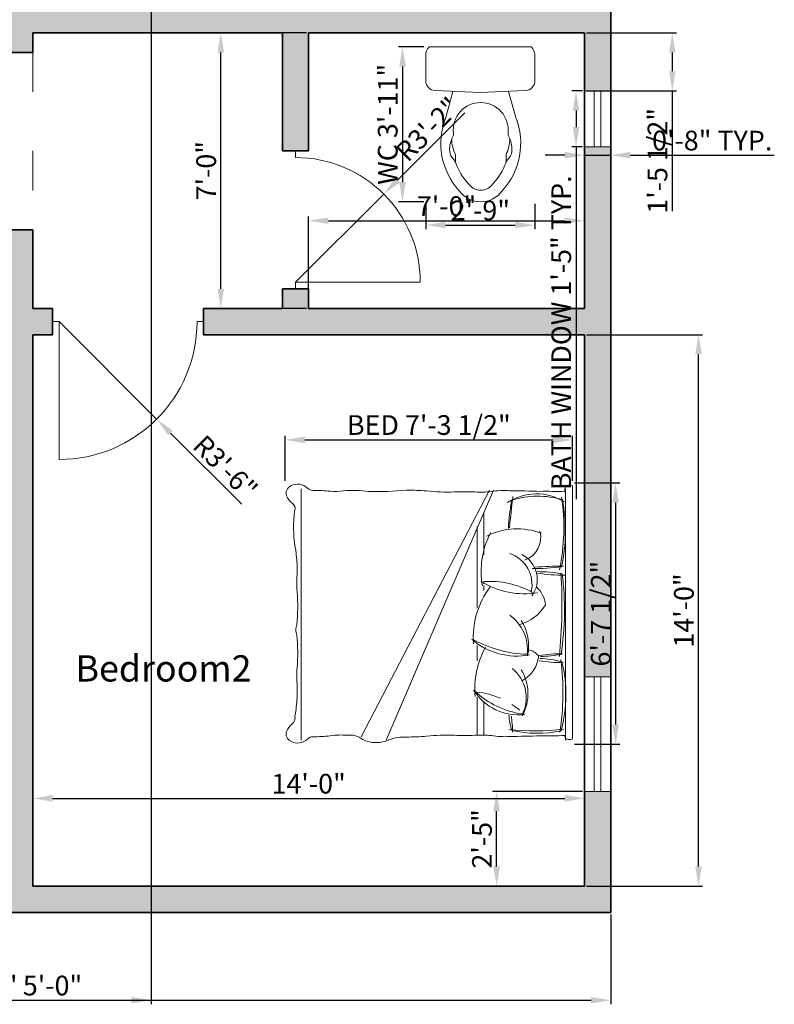
# Model space of a CAD drawing. Units: inches. Extents: x 2129 to 3258, y 1851 to 3021.
# Tile 4 of 10: x 2390 to 2620, y 1851 to 2151. Entities that reach past the tile are written whole.
import ezdxf

# ---------------------------------------------------------------- set-up
doc = ezdxf.new("R2010")
doc.units = ezdxf.units.IN
doc.linetypes.add('ACAD_ISO03W100', pattern=[30, 12, -18])
for name, color, linetype, lineweight in [('A-ANNO-DIMS', 2, 'Continuous', 18), ('A-AREA-IDEN', 7, 'Continuous', 20), ('A-DOOR', 4, 'Continuous', 18), ('A-FLOR-FIXT', 9, 'Continuous', 18), ('A-FURN', 8, 'Continuous', 18), ('A-GLAZ', 4, 'Continuous', 18), ('A-WALL', 7, 'Continuous', 35), ('A-WALL-OVHD', 8, 'ACAD_ISO03W100', 18)]:
    doc.layers.add(name, color=color, linetype=linetype, lineweight=lineweight)
doc.layers.add('A-WALL-PATT', color=32, linetype='Continuous', lineweight=13, true_color=0xcd6928)
doc.styles.get("Standard").update_dxf_attribs({"font": 'arial.ttf'})
doc.dimstyles.new('ISO-25', dxfattribs={"dimtxt": 6, "dimasz": 6, "dimexe": 1.25, "dimexo": 0.625, "dimtad": 1, "dimdec": 1, "dimlunit": 3, "dimtxsty": 'Standard', "dimcen": 2.5, "dimclrd": 5, "dimclre": 5, "dimadec": 0, "dimazin": 0, "dimtfac": 1, "dimtdec": 1, "dimtmove": 0, "dimatfit": 3, "dimfxl": 1, "dimarcsym": 0})

# ---------------------------------------------------------------- blocks, each defined once
blk = doc.blocks.new('bed 1- king size')
at = {"color": 0}
for p, q in [((-0.9487, -0.0777), (0.9323, -0.0777)), ((-0.9394, -0.6151), (0.9323, -1.4177)), ((-0.9394, -0.6451), (0.9066, -1.6065)), ((-0.7682, -0.6873), (-0.4547, -0.6873)), ((-0.2254, -0.6873), (-0.1884, -0.6873)), ((0.6495, -0.6873), (0.8951, -0.6873)), ((-0.6659, -0.7381), (-0.0555, -0.7381)), ((0.2254, -0.7381), (0.3384, -0.7381)), ((0.6103, -0.7381), (0.8953, -0.7381)), ((-0.9487, -2.0547), (0.9323, -2.0547))]:
    blk.add_line(p, q, dxfattribs=at)
blk.add_lwpolyline([(0.898, -0.0829, 0.098699), (0.9236, -0.072, 0.222522), (0.9236, -0.0243), (-0.9705, -0.0243, 0.171621), (-0.9716, -0.0739, 0.102495), (-0.9268, -0.0829, 0.015571), (-0.9293, -0.2659, 0.00267), (-0.9341, -0.4944, 0.058958), (-0.9274, -0.6315, -0.038458), (-0.9248, -0.7552, 0.025508), (-0.9248, -0.9094, -0.039412), (-0.9326, -1.1154, 0.016498), (-0.9382, -1.2654, -0.035771), (-0.9288, -1.5502, 0.045388), (-0.9341, -1.7389, -0.080578), (-0.9295, -1.837, 0.026504), (-0.9362, -1.9656, -0.211134), (-0.9531, -2.0066, 0.329446), (-0.9701, -2.1314, 0.37589), (-0.8958, -2.1647, 0.123892), (-0.8425, -2.1233, -0.342539), (-0.78, -2.1029, 0.07104), (-0.5197, -2.1004, -0.036442), (-0.3847, -2.0853, -0.046791), (-0.2759, -2.0873, 0.023628), (-0.1759, -2.0852, -0.055897), (0.0662, -2.0877, 0.053528), (0.1067, -2.0945, 0.053528), (0.1472, -2.0877, -0.055897), (0.3893, -2.0852, 0.026973), (0.4769, -2.0873, -0.036947), (0.6147, -2.0853, -0.036442), (0.7497, -2.1004, -0.281256), (0.8137, -2.1233, -0.521995), (0.8137, -2.1233, 0.123892), (0.867, -2.1647, 0.37589), (0.9413, -2.1314, 0.329446), (0.9243, -2.0066, -0.211134), (0.9074, -1.9656, 0.026504), (0.9007, -1.837, -0.06219), (0.896, -1.7098, -0.218233), (0.9286, -1.5937, 0.123513), (0.9499, -1.4937, 0.129887), (0.9293, -1.3978, -0.095063), (0.9094, -1.2654, 0.016498), (0.9038, -1.1154, -0.039412), (0.896, -0.9094, 0.025508), (0.896, -0.7552, -0.038458), (0.8986, -0.6315, 0.058958), (0.9053, -0.4944, 0.00267), (0.9005, -0.2659, 0.015571)], format="xyb", close=True, dxfattribs=at)
for centre, radius, start, end in [((0.5931, -1.1167), 1.0433, 75.01813, 103.73916), ((-0.5221, -0.2938), 0.3887, 147.50996, 213.83359), ((-0.2311, -0.2827), 0.6619, 163.92635, 197.14087), ((-0.6569, -1.6774), 1.5884, 78.54853, 98.3029), ((-0.6323, -1.3651), 1.2872, 78.01421, 100.51248), ((2.5431, -0.0869), 2.9129, 180.10628, 184.33117), ((-1.857, -0.3037), 1.5051, 359.15358, 7.55329), ((0.7071, -0.2897), 1.0355, 169.53013, 179.93405), ((-1.2482, -0.1161), 0.9455, 349.58899, 2.04467), ((-0.0818, -4.0689), 3.9654, 84.36579, 93.39687), ((-0.04, -2.1818), 2.0978, 80.93396, 97.42659), ((1.0242, -0.1263), 0.7375, 177.82608, 191.47674), ((-0.6896, -0.2953), 0.9974, 1.8337, 10.6945), ((1.0572, -0.2894), 0.7358, 165.3434, 178.38757), ((0.5721, -2.1074), 2.0115, 81.37136, 96.91703), ((-0.3946, -0.1329), 0.7459, 349.16666, 3.12297), ((-1.0492, -0.3038), 1.9129, 354.09351, 6.47074), ((0.0089, -0.2863), 0.8722, 347.31751, 11.74345), ((-0.1358, -0.4371), 0.5128, 159.30257, 206.50263), ((-0.5846, -0.4421), 0.1803, 18.93869, 104.67251), ((-0.2688, -0.4962), 0.2082, 54.16706, 153.84213), ((-0.7873, -0.3825), 0.6248, 328.65419, 9.19769), ((-0.0546, -0.4435), 0.2189, 96.89924, 136.04208), ((-0.2438, -0.5051), 0.323, 15.40176, 59.7122), ((0.347, -0.3604), 0.0899, 120.11341, 175.89742), ((0.2786, -0.5137), 0.2374, 28.19956, 86.50605), ((-0.2301, -0.5756), 0.2484, 78.04126, 160.83423), ((0.4039, -0.6426), 0.6595, 151.04555, 184.14969), ((0.2545, -0.6795), 0.3178, 83.56066, 144.28529), ((0.2294, -0.7137), 0.3612, 78.40806, 122.00775), ((-0.2123, -0.4404), 0.5157, 319.13389, 10.52989), ((-0.5982, -0.336), 0.8889, 331.60495, 358.1749), ((0.5856, -0.7025), 0.345, 61.64039, 121.33448), ((0.6148, -0.6485), 0.2783, 61.88763, 141.87071), ((0.3458, -0.4294), 0.3969, 302.32623, 7.00001), ((0.0793, -0.3025), 0.6649, 317.32013, 351.4624), ((1.163, -0.8025), 0.5939, 139.95083, 146.95102), ((-1.8444, -10.4721), 10.046, 83.21322, 84.54762), ((-0.6059, 0.7469), 1.2515, 258.11692, 267.88493), ((0.6944, 0.0492), 0.5523, 275.44698, 287.41987), ((0.8799, -1.1936), 0.7214, 90.64318, 100.27066), ((1.163, -0.8025), 0.5939, 156.29818, 173.85386), ((-0.3293, -0.0779), 0.6301, 242.38587, 279.89508), ((0.1632, -0.137), 0.6293, 233.2201, 274.49725), ((0.5459, -0.118), 0.637, 240.94673, 275.46705)]:
    blk.add_arc(centre, radius, start, end, dxfattribs=at)
blk = doc.blocks.new('A$C1308471B')
at = {"ltscale": 20}
for p, q in [((0.0354, 0.4793), (0.1495, 0.4793)), ((0, 0.4607), (0, 0.0186)), ((0.2013, 0.2397), (0.1923, 0.4384)), ((0.1957, 0.3639), (0.3109, 0.3953)), ((0.5021, 0.3528), (0.4724, 0.3528)), ((0.4982, 0.3575), (0.4822, 0.3709)), ((0.2013, 0.2397), (0.1923, 0.0409)), ((0.5021, 0.1304), (0.4724, 0.1304)), ((0.1959, 0.1193), (0.3109, 0.0879)), ((0.4982, 0.1257), (0.4822, 0.1123)), ((0.0354, 0), (0.1495, 0))]:
    blk.add_line(p, q, dxfattribs=at)
for centre, radius, start, end in [((0.0354, 0.4328), 0.0465, 90, 136.5269), ((0.1495, 0.4365), 0.0429, 2.5755, 90), ((0.006, 0.4607), 0.006, 136.5269, 180), ((0.4248, 0.1104), 0.3068, 47.4135, 111.7924), ((0.3654, 0.2416), 0.1206, 83.3523, 180), ((0.3823, 0.3868), 0.0255, 263.3523, 298.5742), ((0.4494, 0.2636), 0.1148, 79.3968, 118.5742), ((0.405, 0.2159), 0.153, 63.502, 90.4522), ((0.4658, 0.3513), 0.0255, 50, 79.3968), ((0.5146, 0.377), 0.0255, 230, 251.3881), ((0.5021, 0.3273), 0.0255, 70.3751, 90), ((0.4248, 0.1104), 0.2558, 46.612, 70.3751), ((0.5654, 0.2416), 0.116, 0, 54.7115), ((0.5654, 0.2416), 0.065, 0, 57.2974), ((0.3654, 0.2416), 0.1206, 180, 276.6477), ((0.5654, 0.2416), 0.065, 302.7026, 0), ((0.5654, 0.2416), 0.116, 305.2885, 0), ((0.4248, 0.3728), 0.2558, 289.6249, 313.388), ((0.4248, 0.3728), 0.3068, 248.2076, 312.5865), ((0.405, 0.2673), 0.153, 269.5478, 296.498), ((0.5146, 0.1062), 0.0255, 108.6119, 130), ((0.5021, 0.1559), 0.0255, 270, 289.6249), ((0.3823, 0.0964), 0.0255, 61.4258, 96.6477), ((0.4494, 0.2196), 0.1148, 241.4258, 280.6032), ((0.4658, 0.1319), 0.0255, 280.6032, 310), ((0.006, 0.0186), 0.006, 180, 223.4731), ((0.0354, 0.0465), 0.0465, 223.4731, 270), ((0.1495, 0.0429), 0.0429, 270, 357.4245)]:
    blk.add_arc(centre, radius, start, end, dxfattribs=at)
blk = doc.blocks.new('WIN-PLAN-35')
for p, q in [((0, 5), (35, 5)), ((0, 3), (35, 3))]:
    blk.add_line(p, q)
blk.add_lwpolyline([(0, 8), (35, 8), (35, 0), (0, 0)], close=True)
blk = doc.blocks.new('WIN-PLAN-17')
for p, q in [((0, 5), (17.03, 5)), ((0, 3), (17.03, 3))]:
    blk.add_line(p, q)
blk.add_lwpolyline([(0, 8), (17.03, 8), (17.03, 0), (0, 0)], close=True)
blk = doc.blocks.new('*D64')
at = {"layer": 'A-ANNO-DIMS', "color": 5, "lineweight": -2, "transparency": 16777216}
for p, q in [((2561.3, 2129.53), (2558.12, 2129.53)), ((2559.37, 2123.53), (2559.37, 2118.5)), ((2561.3, 2112.5), (2558.12, 2112.5)), ((2559.37, 2112.5), (2559.37, 2005.15))]:
    blk.add_line(p, q, dxfattribs=at)
at = {"layer": 'A-ANNO-DIMS', "color": 5, "transparency": 16777216}
for points in [[(2558.37, 2123.53), (2560.37, 2123.53), (2559.37, 2129.53)], [(2558.37, 2118.5), (2560.37, 2118.5), (2559.37, 2112.5)]]:
    blk.add_solid(points, dxfattribs=at)
at = {"layer": 'Defpoints', "color": 0, "transparency": 16777216}
for p in [(2561.93, 2129.53), (2559.37, 2112.5), (2561.93, 2112.5)]:
    blk.add_point(p, dxfattribs=at)
at = {"layer": 'A-ANNO-DIMS', "color": 0, "transparency": 16777216, "insert": (2555.64, 2055.83), "char_height": 6, "attachment_point": 5, "rotation": 90}
blk.add_mtext('BATH WINDOW 1\'-5" TYP.', dxfattribs=at)
blk = doc.blocks.new('*D65')
at = {"layer": 'A-ANNO-DIMS', "color": 5, "lineweight": -2, "transparency": 16777216}
for p, q in [((2555.93, 2109.95), (2549.93, 2109.95)), ((2561.93, 2111.88), (2561.93, 2108.7)), ((2561.93, 2109.95), (2569.93, 2109.95)), ((2569.93, 2111.88), (2569.93, 2108.7)), ((2575.93, 2109.95), (2619.75, 2109.95))]:
    blk.add_line(p, q, dxfattribs=at)
at = {"layer": 'A-ANNO-DIMS', "color": 5, "transparency": 16777216}
for points in [[(2555.93, 2110.95), (2555.93, 2108.95), (2561.93, 2109.95)], [(2575.93, 2110.95), (2575.93, 2108.95), (2569.93, 2109.95)]]:
    blk.add_solid(points, dxfattribs=at)
at = {"layer": 'Defpoints', "color": 0, "transparency": 16777216}
for p in [(2561.93, 2112.5), (2569.93, 2112.5), (2569.93, 2109.95)]:
    blk.add_point(p, dxfattribs=at)
at = {"layer": 'A-ANNO-DIMS', "color": 0, "transparency": 16777216, "insert": (2600.84, 2113.63), "char_height": 6, "attachment_point": 5}
blk.add_mtext('0\'-8" TYP.', dxfattribs=at)
blk = doc.blocks.new('*D66')
at = {"layer": 'A-ANNO-DIMS', "color": 5, "lineweight": -2, "transparency": 16777216}
for p, q in [((2470.78, 2010.72), (2470.78, 2024.47)), ((2476.78, 2023.22), (2552.29, 2023.22)), ((2558.29, 2010.72), (2558.29, 2024.47))]:
    blk.add_line(p, q, dxfattribs=at)
at = {"layer": 'A-ANNO-DIMS', "color": 5, "transparency": 16777216}
for points in [[(2476.78, 2024.22), (2476.78, 2022.22), (2470.78, 2023.22)], [(2552.29, 2024.22), (2552.29, 2022.22), (2558.29, 2023.22)]]:
    blk.add_solid(points, dxfattribs=at)
at = {"layer": 'Defpoints', "color": 0, "transparency": 16777216}
for p in [(2558.29, 2023.22), (2470.78, 2010.09), (2558.29, 2010.09)]:
    blk.add_point(p, dxfattribs=at)
at = {"layer": 'A-ANNO-DIMS', "color": 0, "transparency": 16777216, "insert": (2514.54, 2026.95), "char_height": 6, "attachment_point": 5}
blk.add_mtext('BED 7\'-3 1/2"', dxfattribs=at)
blk = doc.blocks.new('*D67')
at = {"layer": 'A-ANNO-DIMS', "color": 5, "lineweight": -2, "transparency": 16777216}
for p, q in [((2558.92, 2010.09), (2572.67, 2010.09)), ((2571.42, 2004.09), (2571.42, 1936.46)), ((2558.92, 1930.46), (2572.67, 1930.46))]:
    blk.add_line(p, q, dxfattribs=at)
at = {"layer": 'A-ANNO-DIMS', "color": 5, "transparency": 16777216}
for points in [[(2570.42, 2004.09), (2572.42, 2004.09), (2571.42, 2010.09)], [(2570.42, 1936.46), (2572.42, 1936.46), (2571.42, 1930.46)]]:
    blk.add_solid(points, dxfattribs=at)
at = {"layer": 'Defpoints', "color": 0, "transparency": 16777216}
for p in [(2558.29, 2010.09), (2558.29, 1930.46), (2571.42, 1930.46)]:
    blk.add_point(p, dxfattribs=at)
at = {"layer": 'A-ANNO-DIMS', "color": 0, "transparency": 16777216, "insert": (2567.69, 1970.27), "char_height": 6, "attachment_point": 5, "rotation": 90}
blk.add_mtext('6\'-7 1/2"', dxfattribs=at)
blk = doc.blocks.new('*D72')
at = {"layer": 'A-ANNO-DIMS', "color": 5, "lineweight": -2, "transparency": 16777216}
for p, q in [((2512.98, 2142.97), (2505.27, 2142.97)), ((2506.52, 2136.97), (2506.52, 2101.74)), ((2512.98, 2095.74), (2505.27, 2095.74))]:
    blk.add_line(p, q, dxfattribs=at)
at = {"layer": 'A-ANNO-DIMS', "color": 5, "transparency": 16777216}
for points in [[(2505.52, 2136.97), (2507.52, 2136.97), (2506.52, 2142.97)], [(2505.52, 2101.74), (2507.52, 2101.74), (2506.52, 2095.74)]]:
    blk.add_solid(points, dxfattribs=at)
at = {"layer": 'Defpoints', "color": 0, "transparency": 16777216}
for p in [(2513.6, 2142.97), (2506.52, 2095.74), (2513.6, 2095.74)]:
    blk.add_point(p, dxfattribs=at)
at = {"layer": 'A-ANNO-DIMS', "color": 0, "transparency": 16777216, "insert": (2502.79, 2119.36), "char_height": 6, "attachment_point": 5, "rotation": 90}
blk.add_mtext('WC 3\'-11"', dxfattribs=at)
blk = doc.blocks.new('*D73')
at = {"layer": 'A-ANNO-DIMS', "color": 5, "lineweight": -2, "transparency": 16777216}
for p, q in [((2513.6, 2095.11), (2513.6, 2087.4)), ((2546.83, 2095.11), (2546.83, 2087.4)), ((2519.6, 2088.65), (2540.83, 2088.65))]:
    blk.add_line(p, q, dxfattribs=at)
at = {"layer": 'A-ANNO-DIMS', "color": 5, "transparency": 16777216}
for points in [[(2519.6, 2089.65), (2519.6, 2087.65), (2513.6, 2088.65)], [(2540.83, 2089.65), (2540.83, 2087.65), (2546.83, 2088.65)]]:
    blk.add_solid(points, dxfattribs=at)
at = {"layer": 'Defpoints', "color": 0, "transparency": 16777216}
for p in [(2513.6, 2095.74), (2546.83, 2095.74), (2546.83, 2088.65)]:
    blk.add_point(p, dxfattribs=at)
at = {"layer": 'A-ANNO-DIMS', "color": 0, "transparency": 16777216, "insert": (2530.22, 2092.34), "char_height": 6, "attachment_point": 5}
blk.add_mtext('2\'-9"', dxfattribs=at)
blk = doc.blocks.new('*D86')
at = {"layer": 'A-ANNO-DIMS', "color": 5, "lineweight": -2, "transparency": 16777216}
for p, q in [((2185.93, 1878.61), (2185.93, 1851.23)), ((2569.93, 1878.61), (2569.93, 1851.23)), ((2191.93, 1852.48), (2563.93, 1852.48))]:
    blk.add_line(p, q, dxfattribs=at)
at = {"layer": 'A-ANNO-DIMS', "color": 5, "transparency": 16777216}
for points in [[(2191.93, 1853.48), (2191.93, 1851.48), (2185.93, 1852.48)], [(2563.93, 1853.48), (2563.93, 1851.48), (2569.93, 1852.48)]]:
    blk.add_solid(points, dxfattribs=at)
at = {"layer": 'Defpoints', "color": 0, "transparency": 16777216}
for p in [(2185.93, 1879.23), (2569.93, 1879.23), (2569.93, 1852.48)]:
    blk.add_point(p, dxfattribs=at)
at = {"layer": 'A-ANNO-DIMS', "color": 0, "transparency": 16777216, "insert": (2377.93, 1856.18), "char_height": 6, "attachment_point": 5}
blk.add_mtext('32\'-0"', dxfattribs=at)
blk = doc.blocks.new('*D87')
at = {"layer": 'A-ANNO-DIMS', "color": 5, "lineweight": -2, "transparency": 16777216}
for p, q in [((2393.93, 1887.86), (2393.93, 1915.23)), ((2561.93, 1887.86), (2561.93, 1915.23)), ((2399.93, 1913.98), (2555.93, 1913.98))]:
    blk.add_line(p, q, dxfattribs=at)
at = {"layer": 'A-ANNO-DIMS', "color": 5, "transparency": 16777216}
for points in [[(2399.93, 1914.98), (2399.93, 1912.98), (2393.93, 1913.98)], [(2555.93, 1914.98), (2555.93, 1912.98), (2561.93, 1913.98)]]:
    blk.add_solid(points, dxfattribs=at)
at = {"layer": 'Defpoints', "color": 0, "transparency": 16777216}
for p in [(2561.93, 1913.98), (2393.93, 1887.23), (2561.93, 1887.23)]:
    blk.add_point(p, dxfattribs=at)
at = {"layer": 'A-ANNO-DIMS', "color": 0, "transparency": 16777216, "insert": (2477.93, 1917.67), "char_height": 6, "attachment_point": 5}
blk.add_mtext('14\'-0"', dxfattribs=at)
blk = doc.blocks.new('*D88')
at = {"layer": 'A-ANNO-DIMS', "color": 5, "lineweight": -2, "transparency": 16777216}
for p, q in [((2562.55, 2055.23), (2597.93, 2055.23)), ((2596.68, 1893.23), (2596.68, 2049.23)), ((2562.55, 1887.23), (2597.93, 1887.23))]:
    blk.add_line(p, q, dxfattribs=at)
at = {"layer": 'A-ANNO-DIMS', "color": 5, "transparency": 16777216}
for points in [[(2595.68, 2049.23), (2597.68, 2049.23), (2596.68, 2055.23)], [(2595.68, 1893.23), (2597.68, 1893.23), (2596.68, 1887.23)]]:
    blk.add_solid(points, dxfattribs=at)
at = {"layer": 'Defpoints', "color": 0, "transparency": 16777216}
for p in [(2561.93, 2055.23), (2596.68, 2055.23), (2561.93, 1887.23)]:
    blk.add_point(p, dxfattribs=at)
at = {"layer": 'A-ANNO-DIMS', "color": 0, "transparency": 16777216, "insert": (2592.99, 1971.23), "char_height": 6, "attachment_point": 5, "rotation": 90}
blk.add_mtext('14\'-0"', dxfattribs=at)
blk = doc.blocks.new('*D89')
at = {"layer": 'A-ANNO-DIMS', "color": 5, "lineweight": -2, "transparency": 16777216}
for p, q in [((2477.93, 2063.86), (2477.93, 2091.23)), ((2561.93, 2063.86), (2561.93, 2091.23)), ((2483.93, 2089.98), (2555.93, 2089.98))]:
    blk.add_line(p, q, dxfattribs=at)
at = {"layer": 'A-ANNO-DIMS', "color": 5, "transparency": 16777216}
for points in [[(2483.93, 2090.98), (2483.93, 2088.98), (2477.93, 2089.98)], [(2555.93, 2090.98), (2555.93, 2088.98), (2561.93, 2089.98)]]:
    blk.add_solid(points, dxfattribs=at)
at = {"layer": 'Defpoints', "color": 0, "transparency": 16777216}
for p in [(2561.93, 2089.98), (2477.93, 2063.23), (2561.93, 2063.23)]:
    blk.add_point(p, dxfattribs=at)
at = {"layer": 'A-ANNO-DIMS', "color": 0, "transparency": 16777216, "insert": (2519.93, 2093.67), "char_height": 6, "attachment_point": 5}
blk.add_mtext('7\'-0"', dxfattribs=at)
blk = doc.blocks.new('*D90')
at = {"layer": 'A-ANNO-DIMS', "color": 5, "lineweight": -2, "transparency": 16777216}
for p, q in [((2477.3, 2147.23), (2449.93, 2147.23)), ((2451.18, 2069.23), (2451.18, 2141.23)), ((2477.3, 2063.23), (2449.93, 2063.23))]:
    blk.add_line(p, q, dxfattribs=at)
at = {"layer": 'A-ANNO-DIMS', "color": 5, "transparency": 16777216}
for points in [[(2450.18, 2141.23), (2452.18, 2141.23), (2451.18, 2147.23)], [(2450.18, 2069.23), (2452.18, 2069.23), (2451.18, 2063.23)]]:
    blk.add_solid(points, dxfattribs=at)
at = {"layer": 'Defpoints', "color": 0, "transparency": 16777216}
for p in [(2451.18, 2147.23), (2477.93, 2147.23), (2477.93, 2063.23)]:
    blk.add_point(p, dxfattribs=at)
at = {"layer": 'A-ANNO-DIMS', "color": 0, "transparency": 16777216, "insert": (2447.49, 2105.23), "char_height": 6, "attachment_point": 5, "rotation": 90}
blk.add_mtext('7\'-0"', dxfattribs=at)
blk = doc.blocks.new('*D91')
at = {"layer": 'A-ANNO-DIMS', "color": 5, "lineweight": -2, "transparency": 16777216}
for p, q in [((2369.93, 2314.61), (2369.93, 1851.23)), ((2429.93, 2314.61), (2429.93, 1851.23)), ((2375.93, 1852.48), (2423.93, 1852.48))]:
    blk.add_line(p, q, dxfattribs=at)
at = {"layer": 'A-ANNO-DIMS', "color": 5, "transparency": 16777216}
for points in [[(2375.93, 1853.48), (2375.93, 1851.48), (2369.93, 1852.48)], [(2423.93, 1853.48), (2423.93, 1851.48), (2429.93, 1852.48)]]:
    blk.add_solid(points, dxfattribs=at)
at = {"layer": 'Defpoints', "color": 0, "transparency": 16777216}
for p in [(2369.93, 2315.23), (2429.93, 2315.23), (2429.93, 1852.48)]:
    blk.add_point(p, dxfattribs=at)
at = {"layer": 'A-ANNO-DIMS', "color": 0, "transparency": 16777216, "insert": (2399.93, 1856.17), "char_height": 6, "attachment_point": 5}
blk.add_mtext('5\'-0"', dxfattribs=at)
blk = doc.blocks.new('*D112')
at = {"layer": 'A-ANNO-DIMS', "color": 5, "lineweight": -2, "transparency": 16777216}
for p, q in [((2561.3, 1916.04), (2533.93, 1916.04)), ((2535.18, 1893.23), (2535.18, 1910.04)), ((2561.3, 1887.23), (2533.93, 1887.23))]:
    blk.add_line(p, q, dxfattribs=at)
at = {"layer": 'A-ANNO-DIMS', "color": 5, "transparency": 16777216}
for points in [[(2534.18, 1910.04), (2536.18, 1910.04), (2535.18, 1916.04)], [(2534.18, 1893.23), (2536.18, 1893.23), (2535.18, 1887.23)]]:
    blk.add_solid(points, dxfattribs=at)
at = {"layer": 'Defpoints', "color": 0, "transparency": 16777216}
for p in [(2535.18, 1916.04), (2561.93, 1916.04), (2561.93, 1887.23)]:
    blk.add_point(p, dxfattribs=at)
at = {"layer": 'A-ANNO-DIMS', "color": 0, "transparency": 16777216, "insert": (2531.49, 1901.64), "char_height": 6, "attachment_point": 5, "rotation": 90}
blk.add_mtext('2\'-5"', dxfattribs=at)
blk = doc.blocks.new('*D114')
at = {"layer": 'A-ANNO-DIMS', "color": 5, "lineweight": -2, "transparency": 16777216}
for p, q in [((2562.55, 2147.23), (2589.93, 2147.23)), ((2588.68, 2141.23), (2588.68, 2135.53)), ((2562.55, 2129.53), (2589.93, 2129.53)), ((2588.68, 2129.53), (2588.68, 2092.92))]:
    blk.add_line(p, q, dxfattribs=at)
at = {"layer": 'A-ANNO-DIMS', "color": 5, "transparency": 16777216}
for points in [[(2587.68, 2141.23), (2589.68, 2141.23), (2588.68, 2147.23)], [(2587.68, 2135.53), (2589.68, 2135.53), (2588.68, 2129.53)]]:
    blk.add_solid(points, dxfattribs=at)
at = {"layer": 'Defpoints', "color": 0, "transparency": 16777216}
for p in [(2561.93, 2147.23), (2561.93, 2129.53), (2588.68, 2129.53)]:
    blk.add_point(p, dxfattribs=at)
at = {"layer": 'A-ANNO-DIMS', "color": 0, "transparency": 16777216, "insert": (2584.95, 2108.23), "char_height": 6, "attachment_point": 5, "rotation": 90}
blk.add_mtext('1\'-5 1/2"', dxfattribs=at)
blk = doc.blocks.new('*D136')
at = {"layer": 'A-ANNO-DIMS', "color": 5, "lineweight": -2, "transparency": 16777216}
for p, q in [((2401.93, 2059.23), (2431.63, 2029.54)), ((2457.56, 2003.61), (2435.87, 2025.29))]:
    blk.add_line(p, q, dxfattribs=at)
at = {"layer": 'A-ANNO-DIMS', "color": 5, "transparency": 16777216}
blk.add_solid([(2436.58, 2026), (2435.16, 2024.59), (2431.63, 2029.54)], dxfattribs=at)
at = {"layer": 'Defpoints', "color": 0, "transparency": 16777216}
for p in [(2401.93, 2059.23), (2431.63, 2029.54)]:
    blk.add_point(p, dxfattribs=at)
at = {"layer": 'A-ANNO-DIMS', "color": 0, "transparency": 16777216, "insert": (2452.05, 2014.33), "char_height": 6, "attachment_point": 5, "rotation": 314.9994}
blk.add_mtext('R3\'-6"', dxfattribs=at)
blk = doc.blocks.new('*D137')
at = {"layer": 'A-ANNO-DIMS', "color": 5, "lineweight": -2, "transparency": 16777216}
for p, q in [((2525.51, 2122.81), (2505.04, 2102.35)), ((2473.93, 2071.23), (2500.8, 2098.1))]:
    blk.add_line(p, q, dxfattribs=at)
at = {"layer": 'A-ANNO-DIMS', "color": 5, "transparency": 16777216}
blk.add_solid([(2504.33, 2103.05), (2505.75, 2101.64), (2500.8, 2098.1)], dxfattribs=at)
at = {"layer": 'Defpoints', "color": 0, "transparency": 16777216}
for p in [(2500.8, 2098.1), (2473.93, 2071.23)]:
    blk.add_point(p, dxfattribs=at)
at = {"layer": 'A-ANNO-DIMS', "color": 0, "transparency": 16777216, "insert": (2514.78, 2117.31), "char_height": 6, "attachment_point": 5, "rotation": 45.0004}
blk.add_mtext('R3\'-2"', dxfattribs=at)

msp = doc.modelspace()

# ---------------------------------------------------------------- hatches: boundary and pattern name
at = {"layer": 'A-WALL-PATT'}
h = msp.add_hatch(color=256, dxfattribs=at)
h.dxf.hatch_style = 1
h.paths.add_polyline_path([(2393.39, 2407.23), (2185.93, 2407.23), (2185.93, 2394.06), (2193.93, 2394.06), (2193.93, 2399.23), (2361.93, 2399.23), (2361.93, 2355.23), (2361.93, 2347.23), (2361.93, 2258.25), (2369.93, 2258.25), (2369.93, 2307.23), (2429.93, 2307.23), (2429.93, 2303.23), (2437.93, 2303.23), (2437.93, 2327.23), (2429.93, 2327.23), (2429.93, 2315.23), (2369.93, 2315.23), (2369.93, 2399.23), (2393.39, 2399.23)])
h.paths.add_polyline_path([(2569.93, 2407.23), (2410.42, 2407.23), (2410.42, 2399.23), (2429.93, 2399.23), (2429.93, 2351.23), (2437.93, 2351.23), (2437.93, 2399.23), (2561.93, 2399.23), (2561.93, 2317.22), (2569.93, 2317.22)])
h.paths.add_polyline_path([(2569.93, 2282.22), (2561.93, 2282.22), (2561.93, 2243.23), (2437.93, 2243.23), (2437.93, 2249.23), (2429.93, 2249.23), (2429.93, 2235.23), (2561.93, 2235.23), (2561.93, 2155.23), (2379.93, 2155.23), (2379.93, 2147.23), (2385.93, 2147.23), (2385.93, 2141.23), (2393.93, 2141.23), (2393.93, 2147.23), (2469.93, 2147.23), (2469.93, 2111.23), (2477.93, 2111.23), (2477.93, 2147.23), (2561.93, 2147.23), (2561.93, 2129.53), (2569.93, 2129.53)])
h.paths.add_polyline_path([(2569.93, 2112.5), (2561.93, 2112.5), (2561.93, 2063.23), (2477.93, 2063.23), (2477.93, 2069.23), (2469.93, 2069.23), (2469.93, 2063.23), (2445.93, 2063.23), (2445.93, 2055.23), (2561.93, 2055.23), (2561.93, 1951.04), (2569.93, 1951.04)])
h.paths.add_polyline_path([(2569.93, 1916.04), (2561.93, 1916.04), (2561.93, 1887.23), (2393.93, 1887.23), (2393.93, 2055.23), (2399.93, 2055.23), (2399.93, 2063.23), (2393.93, 2063.23), (2393.93, 2087.23), (2385.93, 2087.23), (2385.93, 1887.23), (2385.93, 1879.23), (2569.93, 1879.23)])
h.paths.add_polyline_path([(2193.93, 2147.23), (2289.93, 2147.23), (2289.93, 2155.23), (2193.93, 2155.23), (2193.93, 2170.77), (2185.93, 2170.77), (2185.93, 2056.85), (2193.93, 2056.85)])
h.paths.add_polyline_path([(2193.93, 2021.85), (2185.93, 2021.85), (2185.93, 1959.23), (2222.56, 1959.23), (2222.56, 1967.23), (2193.93, 1967.23)])
h.paths.add_polyline_path([(2307.93, 1967.23), (2257.56, 1967.23), (2257.56, 1959.23), (2307.93, 1959.23)])
h.paths.add_polyline_path([(2255.61, 2368.18), (2321.09, 2368.18), (2321.09, 2384.66), (2255.61, 2384.66)], flags=25)
h.paths.add_polyline_path([(2282.89, 2032.34), (2325.27, 2032.34), (2325.27, 2051.27), (2282.89, 2051.27)], flags=9)
h.paths.add_polyline_path([(2404.09, 1945.18), (2463.36, 1945.18), (2463.36, 1961.66), (2404.09, 1961.66)], flags=25)
h.paths.add_polyline_path([(2494.41, 2286.84), (2553.68, 2286.84), (2553.68, 2303.32), (2494.41, 2303.32)], flags=9)
h.paths.add_polyline_path([(2389.71, 2321.98), (2411.09, 2321.98), (2411.09, 2338.47), (2389.71, 2338.47)], flags=25)
h.paths.add_polyline_path([(2219.41, 2162.82), (2258.18, 2162.82), (2258.18, 2179.3), (2219.41, 2179.3)], flags=9)
h.paths.add_polyline_path([(2249.68, 2306.23), (2298.12, 2306.23), (2298.12, 2323.98), (2249.68, 2323.98)], flags=25)
h = msp.add_hatch(color=256, dxfattribs=at)
h.dxf.hatch_style = 1
h.paths.add_polyline_path([(2193.93, 2288.35), (2185.93, 2288.35), (2185.93, 2205.77), (2193.93, 2205.77)])
h.paths.add_polyline_path([(2193.93, 2347.23), (2310.77, 2347.23), (2310.77, 2355.23), (2193.93, 2355.23), (2193.93, 2359.06), (2185.93, 2359.06), (2185.93, 2323.35), (2193.93, 2323.35)])
h.paths.add_polyline_path([(2314.44, 2244.01), (2314.44, 2257.94), (2302.07, 2257.94), (2302.07, 2244.01)], flags=9)
h.paths.add_polyline_path([(2255.61, 2368.18), (2321.09, 2368.18), (2321.09, 2384.66), (2255.61, 2384.66)], flags=9)
h.paths.add_polyline_path([(2282.89, 2032.34), (2325.27, 2032.34), (2325.27, 2051.27), (2282.89, 2051.27)], flags=9)
h.paths.add_polyline_path([(2404.09, 1945.18), (2463.36, 1945.18), (2463.36, 1961.66), (2404.09, 1961.66)], flags=9)
h.paths.add_polyline_path([(2494.41, 2286.84), (2553.68, 2286.84), (2553.68, 2303.32), (2494.41, 2303.32)], flags=9)
h.paths.add_polyline_path([(2389.71, 2321.98), (2411.09, 2321.98), (2411.09, 2338.47), (2389.71, 2338.47)], flags=9)
h.paths.add_polyline_path([(2219.41, 2162.82), (2258.18, 2162.82), (2258.18, 2179.3), (2219.41, 2179.3)], flags=9)
h.paths.add_polyline_path([(2249.68, 2306.23), (2298.12, 2306.23), (2298.12, 2323.98), (2249.68, 2323.98)], flags=9)

# ---------------------------------------------------------------- linework, layer by layer
at = {"layer": 'A-DOOR'}
for p, q in [((2473.93, 2111.23), (2473.93, 2109.23)), ((2473.93, 2069.23), (2473.93, 2071.23)), ((2473.93, 2071.23), (2511.93, 2071.23)), ((2399.93, 2059.23), (2401.93, 2059.23)), ((2401.93, 2017.23), (2401.93, 2059.23)), ((2445.93, 2059.23), (2443.93, 2059.23))]:
    msp.add_line(p, q, dxfattribs=at)
for centre, radius, start, end in [((2473.93, 2071.23), 38, 0, 90), ((2401.93, 2059.23), 42, 270, 0)]:
    msp.add_arc(centre, radius, start, end, dxfattribs=at)
at = {"layer": 'A-WALL'}
for p, q in [((2393.93, 2147.23), (2469.93, 2147.23)), ((2393.93, 2141.23), (2393.93, 2147.23)), ((2469.93, 2147.23), (2469.93, 2111.23)), ((2477.93, 2147.23), (2477.93, 2111.23)), ((2477.93, 2147.23), (2561.93, 2147.23)), ((2561.93, 2147.23), (2561.93, 2063.23)), ((2385.93, 2141.23), (2393.93, 2141.23)), ((2469.93, 2111.23), (2477.93, 2111.23)), ((2393.93, 2087.23), (2385.93, 2087.23)), ((2393.93, 2063.23), (2393.93, 2087.23)), ((2469.93, 2069.23), (2477.93, 2069.23)), ((2469.93, 2069.23), (2469.93, 2063.23)), ((2477.93, 2069.23), (2477.93, 2063.23)), ((2393.93, 2063.23), (2399.93, 2063.23)), ((2399.93, 2063.23), (2399.93, 2055.23)), ((2445.93, 2063.23), (2445.93, 2055.23)), ((2445.93, 2063.23), (2469.93, 2063.23)), ((2477.93, 2063.23), (2561.93, 2063.23)), ((2393.93, 1887.23), (2393.93, 2055.23)), ((2393.93, 2055.23), (2399.93, 2055.23)), ((2445.93, 2055.23), (2561.93, 2055.23))]:
    msp.add_line(p, q, dxfattribs=at)
msp.add_lwpolyline([(2185.93, 2407.23), (2569.93, 2407.23), (2569.93, 1879.23), (2185.93, 1879.23)], close=True, dxfattribs=at)
for points in [[(2561.93, 2147.23), (2561.93, 2063.23)], [(2561.93, 2055.23), (2561.93, 1887.23), (2393.93, 1887.23)]]:
    msp.add_lwpolyline(points, dxfattribs=at)
at = {"layer": 'A-WALL-OVHD'}
msp.add_line((2393.93, 2141.23), (2393.93, 2087.23), dxfattribs=at)

# ---------------------------------------------------------------- block references
at = {"layer": 'A-FLOR-FIXT', "xscale": 69.32133872191167, "yscale": 69.32133872191167, "zscale": 69.32133872191167, "rotation": 269.9999999999996}
msp.add_blockref('A$C1308471B', (2513.6, 2142.97), dxfattribs=at)
at = {"layer": 'A-FURN', "xscale": 40.71179162366628, "yscale": 40.71179162366628, "zscale": 40.71179162366628, "rotation": 270}
msp.add_blockref('bed 1- king size', (2559.28, 1969.69), dxfattribs=at)
at = {"layer": 'A-GLAZ'}
for name, p, rotation in [('WIN-PLAN-17', (2561.93, 2129.53), 269.9999999999922), ('WIN-PLAN-35', (2569.93, 1916.04), 89.99999999999984)]:
    msp.add_blockref(name, p, dxfattribs=dict(at, rotation=rotation))

# ---------------------------------------------------------------- texts
at = {"layer": 'A-AREA-IDEN', "insert": (2406.91, 1957.58), "char_height": 8, "attachment_point": 1}
msp.add_mtext_dynamic_manual_height_columns('{\\fArial|b1|i0|c0|p34;Bedroom2}', width=58.4293, gutter_width=12.5, heights=[0], dxfattribs=at)

# ---------------------------------------------------------------- dimensions: what is measured, and where the dimension line sits
at = {"layer": 'A-ANNO-DIMS'}
for base, p1, p2, picture, middle in [((2429.93, 1852.48), (2369.93, 2315.23), (2429.93, 2315.23), '*D91', (2399.93, 1856.17)), ((2561.93, 2089.98), (2477.93, 2063.23), (2561.93, 2063.23), '*D89', (2519.93, 2093.67)), ((2546.83, 2088.65), (2513.6, 2095.74), (2546.83, 2095.74), '*D73', (2530.22, 2092.34)), ((2561.93, 1913.98), (2393.93, 1887.23), (2561.93, 1887.23), '*D87', (2477.93, 1917.67)), ((2569.93, 1852.48), (2185.93, 1879.23), (2569.93, 1879.23), '*D86', (2377.93, 1856.18))]:
    dim = msp.add_linear_dim(base=base, p1=p1, p2=p2, dimstyle='ISO-25', override={"dimdec": 1, "dimlfac": 1, "dimrnd": 0, "dimzin": 1, "dimdsep": 46, "dimlunit": 4, "dimfrac": 2}, dxfattribs=at)
    dim.commit()
    dim.dimension.update_dxf_attribs({"geometry": picture, "text_midpoint": middle})
for base, p1, p2, angle, picture, middle in [((2451.18, 2147.23), (2477.93, 2063.23), (2477.93, 2147.23), 90, '*D90', (2447.49, 2105.23)), ((2588.68, 2129.53), (2561.93, 2147.23), (2561.93, 2129.53), 270, '*D114', (2584.95, 2108.23)), ((2596.68, 2055.23), (2561.93, 1887.23), (2561.93, 2055.23), 90, '*D88', (2592.99, 1971.23)), ((2571.42, 1930.46), (2558.29, 2010.09), (2558.29, 1930.46), 270, '*D67', (2567.69, 1970.27)), ((2535.18, 1916.04), (2561.93, 1887.23), (2561.93, 1916.04), 90, '*D112', (2531.49, 1901.64))]:
    dim = msp.add_linear_dim(base=base, p1=p1, p2=p2, angle=angle, dimstyle='ISO-25', override={"dimdec": 1, "dimlfac": 1, "dimrnd": 0, "dimzin": 1, "dimdsep": 46, "dimlunit": 4, "dimfrac": 2}, dxfattribs=at)
    dim.commit()
    dim.dimension.update_dxf_attribs({"geometry": picture, "text_midpoint": middle})
for base, p1, p2, text, picture, middle in [((2506.52, 2095.74), (2513.6, 2142.97), (2513.6, 2095.74), 'WC <>', '*D72', (2502.79, 2119.36)), ((2559.37, 2112.5), (2561.93, 2129.53), (2561.93, 2112.5), 'BATH WINDOW <> TYP.', '*D64', (2555.64, 2055.83))]:
    dim = msp.add_linear_dim(base=base, p1=p1, p2=p2, angle=270, text=text, dimstyle='ISO-25', override={"dimdec": 1, "dimlfac": 1, "dimrnd": 0, "dimzin": 1, "dimdsep": 46, "dimlunit": 4, "dimfrac": 2}, dxfattribs=at)
    dim.commit()
    dim.dimension.update_dxf_attribs({"geometry": picture, "text_midpoint": middle})
dim = msp.add_radius_dim(center=(2473.93, 2071.23), mpoint=(2500.8, 2098.1), dimstyle='ISO-25', override={"dimdec": 1, "dimlfac": 1, "dimrnd": 0, "dimzin": 1, "dimdsep": 46, "dimlunit": 4, "dimfrac": 2}, dxfattribs=at)
dim.commit()
dim.dimension.update_dxf_attribs({"geometry": '*D137', "text_midpoint": (2514.78, 2117.31)})
for base, p1, p2, text, picture, middle in [((2569.93, 2109.95), (2561.93, 2112.5), (2569.93, 2112.5), '<> TYP.', '*D65', (2600.84, 2113.63)), ((2558.29, 2023.22), (2470.78, 2010.09), (2558.29, 2010.09), 'BED <>', '*D66', (2514.54, 2026.95))]:
    dim = msp.add_linear_dim(base=base, p1=p1, p2=p2, text=text, dimstyle='ISO-25', override={"dimdec": 1, "dimlfac": 1, "dimrnd": 0, "dimzin": 1, "dimdsep": 46, "dimlunit": 4, "dimfrac": 2}, dxfattribs=at)
    dim.commit()
    dim.dimension.update_dxf_attribs({"geometry": picture, "text_midpoint": middle})
dim = msp.add_radius_dim(center=(2401.93, 2059.23), mpoint=(2431.63, 2029.54), dimstyle='ISO-25', override={"dimdec": 1, "dimlfac": 1, "dimrnd": 0, "dimzin": 1, "dimdsep": 46, "dimlunit": 4, "dimfrac": 2}, dxfattribs=at)
dim.commit()
dim.dimension.update_dxf_attribs({"geometry": '*D136', "text_midpoint": (2449.45, 2011.72), "dimtype": 164})

doc.saveas('drawing.dxf')
